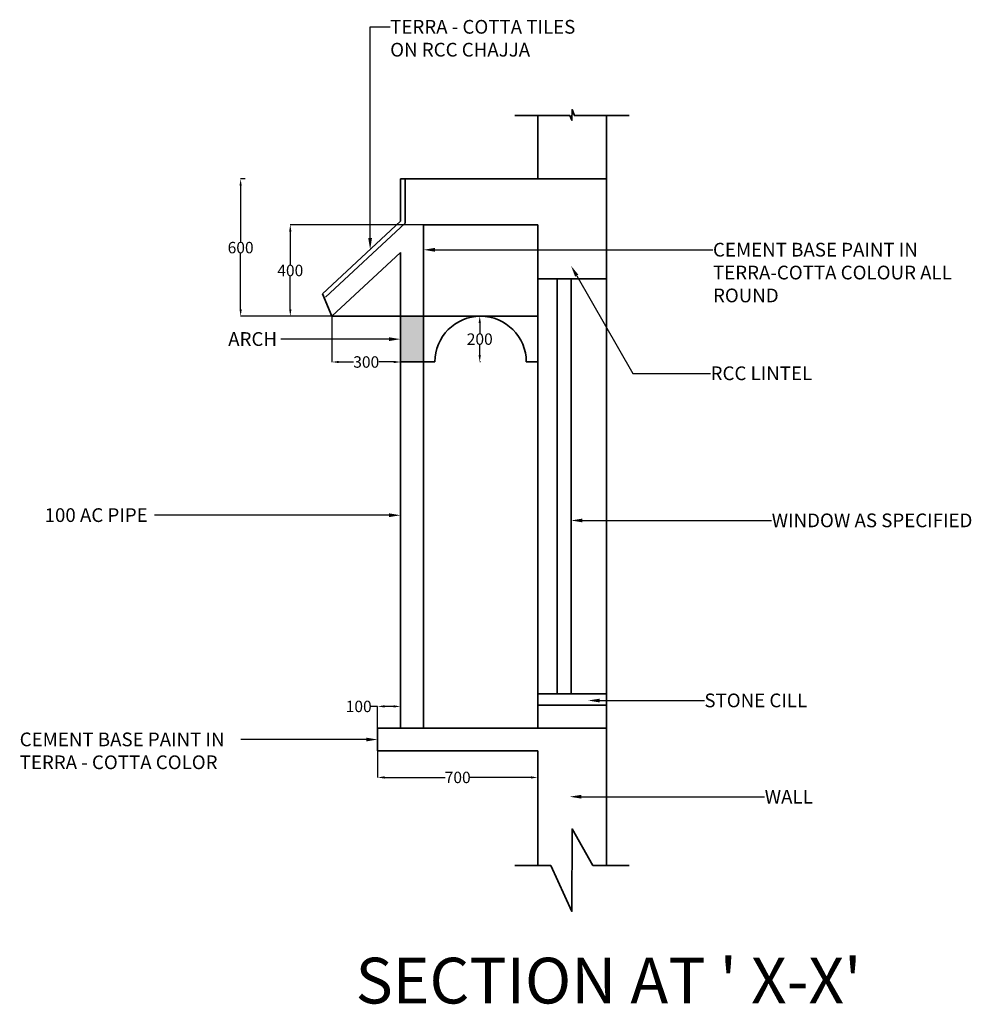
# Model space of a CAD drawing. Units: millimetres. Extents: x 12559 to 31551, y 33148 to 41181.
# Tile 2 of 3: x 19003 to 23164, y 35976 to 40279. Entities that reach past the tile are written whole.
import ezdxf
from ezdxf import colors
from ezdxf.entities.mleader import LeaderData, LeaderLine
from ezdxf.math import Vec2, Vec3

# ---------------------------------------------------------------- set-up
doc = ezdxf.new("R2010")
doc.units = ezdxf.units.MM
doc.header["$MEASUREMENT"] = 0
for name, color, linetype, lineweight in [('A-ANNO-DIMS', 2, 'Continuous', 18), ('A-ANNO-TEXT', 3, 'Continuous', 25), ('A-DETL-PATT', 8, 'Continuous', 13), ('A-SECT', 7, 'Continuous', 35)]:
    doc.layers.add(name, color=color, linetype=linetype, lineweight=lineweight)
doc.styles.get("Standard").update_dxf_attribs({"font": 'arial.ttf'})
doc.dimstyles.get("Standard").update_dxf_attribs({"dimtxt": 100, "dimasz": 0.18, "dimexe": 0.18, "dimexo": 0.0625, "dimgap": 0.09, "dimtad": 0, "dimtih": 1, "dimtoh": 1, "dimdec": 0, "dimzin": 0, "dimdsep": 46, "dimtxsty": 'Standard', "dimcen": 0.09, "dimadec": 0, "dimazin": 0, "dimtfac": 1, "dimtdec": 0, "dimtofl": 0, "dimtmove": 0, "dimatfit": 3, "dimfxl": 1, "dimtolj": 1, "dimtzin": 0, "dimarcsym": 0})

# ---------------------------------------------------------------- blocks, each defined once
blk = doc.blocks.new('*D24')
at = {"layer": 'A-ANNO-DIMS', "color": 0, "lineweight": -2, "transparency": 16777216}
for p, q in [((21018, 38983.1), (21014.3, 38983.1)), ((21014.5, 38953.1), (21014.5, 38908.7)), ((21014.5, 38813.1), (21014.5, 38857.4)), ((21018, 38783.1), (21014.3, 38783.1))]:
    blk.add_line(p, q, dxfattribs=at)
at = {"layer": 'A-ANNO-DIMS', "color": 0, "transparency": 16777216}
for points in [[(21009.5, 38953.1), (21019.5, 38953.1), (21014.5, 38983.1)], [(21009.5, 38813.1), (21019.5, 38813.1), (21014.5, 38783.1)]]:
    blk.add_solid(points, dxfattribs=at)
at = {"layer": 'DEFPOINTS', "color": 0, "transparency": 16777216}
for p in [(21018.1, 38983.1), (21014.5, 38783.1), (21018.1, 38783.1)]:
    blk.add_point(p, dxfattribs=at)
at = {"layer": 'A-ANNO-DIMS', "color": 0, "transparency": 16777216, "insert": (21014.5, 38883.1), "char_height": 50, "attachment_point": 5}
blk.add_mtext('\\A1;200', dxfattribs=at)
blk = doc.blocks.new('*D25')
at = {"layer": 'A-ANNO-DIMS', "color": 0, "lineweight": -2, "transparency": 16777216}
for p, q in [((20368.1, 38983), (20368.1, 38782.9)), ((20668.1, 38983), (20668.1, 38782.9)), ((20398.1, 38783.1), (20462.8, 38783.1)), ((20638.1, 38783.1), (20573.3, 38783.1))]:
    blk.add_line(p, q, dxfattribs=at)
at = {"layer": 'A-ANNO-DIMS', "color": 0, "transparency": 16777216}
for points in [[(20398.1, 38788.1), (20398.1, 38778.1), (20368.1, 38783.1)], [(20638.1, 38788.1), (20638.1, 38778.1), (20668.1, 38783.1)]]:
    blk.add_solid(points, dxfattribs=at)
at = {"layer": 'DEFPOINTS', "color": 0, "transparency": 16777216}
for p in [(20368.1, 38983.1), (20668.1, 38983.1), (20668.1, 38783.1)]:
    blk.add_point(p, dxfattribs=at)
at = {"layer": 'A-ANNO-DIMS', "color": 0, "transparency": 16777216, "insert": (20518.1, 38783.1), "char_height": 50, "attachment_point": 5}
blk.add_mtext('\\A1;300', dxfattribs=at)
blk = doc.blocks.new('*D26')
at = {"layer": 'A-ANNO-DIMS', "color": 0, "lineweight": -2, "transparency": 16777216}
for p, q in [((20768, 39383.1), (20185.8, 39383.1)), ((20186, 39353.1), (20186, 39208.7)), ((20186, 39013.1), (20186, 39157.4)), ((20768, 38983.1), (20185.8, 38983.1))]:
    blk.add_line(p, q, dxfattribs=at)
at = {"layer": 'A-ANNO-DIMS', "color": 0, "transparency": 16777216}
for points in [[(20181, 39353.1), (20191, 39353.1), (20186, 39383.1)], [(20181, 39013.1), (20191, 39013.1), (20186, 38983.1)]]:
    blk.add_solid(points, dxfattribs=at)
at = {"layer": 'DEFPOINTS', "color": 0, "transparency": 16777216}
for p in [(20186, 39383.1), (20768.1, 39383.1), (20768.1, 38983.1)]:
    blk.add_point(p, dxfattribs=at)
at = {"layer": 'A-ANNO-DIMS', "color": 0, "transparency": 16777216, "insert": (20186, 39183.1), "char_height": 50, "attachment_point": 5}
blk.add_mtext('\\A1;400', dxfattribs=at)
blk = doc.blocks.new('*D27')
at = {"layer": 'A-ANNO-DIMS', "color": 0, "lineweight": -2, "transparency": 16777216}
for p, q in [((19988.8, 39583.1), (19968.6, 39583.1)), ((19968.8, 39553.1), (19968.8, 39308.7)), ((19968.8, 39013.1), (19968.8, 39257.4)), ((20185.7, 38983.1), (19968.6, 38983.1))]:
    blk.add_line(p, q, dxfattribs=at)
at = {"layer": 'A-ANNO-DIMS', "color": 0, "transparency": 16777216}
for points in [[(19963.8, 39553.1), (19973.8, 39553.1), (19968.8, 39583.1)], [(19963.8, 39013.1), (19973.8, 39013.1), (19968.8, 38983.1)]]:
    blk.add_solid(points, dxfattribs=at)
at = {"layer": 'DEFPOINTS', "color": 0, "transparency": 16777216}
for p in [(19988.8, 39583.1), (19968.8, 38983.1), (20185.8, 38983.1)]:
    blk.add_point(p, dxfattribs=at)
at = {"layer": 'A-ANNO-DIMS', "color": 0, "transparency": 16777216, "insert": (19968.8, 39283.1), "char_height": 50, "attachment_point": 5}
blk.add_mtext('\\A1;600', dxfattribs=at)
blk = doc.blocks.new('*D28')
at = {"layer": 'A-ANNO-DIMS', "color": 0, "lineweight": -2, "transparency": 16777216}
for p, q in [((20568.1, 37083), (20568.1, 36967.2)), ((21268.1, 37083), (21268.1, 36967.2)), ((20598.1, 36967.4), (20863, 36967.4)), ((21238.1, 36967.4), (20973.1, 36967.4))]:
    blk.add_line(p, q, dxfattribs=at)
at = {"layer": 'A-ANNO-DIMS', "color": 0, "transparency": 16777216}
for points in [[(20598.1, 36972.4), (20598.1, 36962.4), (20568.1, 36967.4)], [(21238.1, 36972.4), (21238.1, 36962.4), (21268.1, 36967.4)]]:
    blk.add_solid(points, dxfattribs=at)
at = {"layer": 'DEFPOINTS', "color": 0, "transparency": 16777216}
for p in [(20568.1, 37083.1), (21268.1, 37083.1), (21268.1, 36967.4)]:
    blk.add_point(p, dxfattribs=at)
at = {"layer": 'A-ANNO-DIMS', "color": 0, "transparency": 16777216, "insert": (20918.1, 36967.4), "char_height": 50, "attachment_point": 5}
blk.add_mtext('\\A1;700', dxfattribs=at)
blk = doc.blocks.new('*D29')
at = {"layer": 'A-ANNO-DIMS', "color": 0, "lineweight": -2, "transparency": 16777216}
for p, q in [((20568.1, 37277.8), (20538.1, 37277.8)), ((20568.1, 37183.1), (20568.1, 37278)), ((20638.1, 37277.8), (20598.1, 37277.8)), ((20668.1, 37183.1), (20668.1, 37278))]:
    blk.add_line(p, q, dxfattribs=at)
at = {"layer": 'A-ANNO-DIMS', "color": 0, "transparency": 16777216}
for points in [[(20598.1, 37282.8), (20598.1, 37272.8), (20568.1, 37277.8)], [(20638.1, 37282.8), (20638.1, 37272.8), (20668.1, 37277.8)]]:
    blk.add_solid(points, dxfattribs=at)
at = {"layer": 'DEFPOINTS', "color": 0, "transparency": 16777216}
for p in [(20568.1, 37277.8), (20568.1, 37183.1), (20668.1, 37183.1)]:
    blk.add_point(p, dxfattribs=at)
at = {"layer": 'A-ANNO-DIMS', "color": 0, "transparency": 16777216, "insert": (20485.2, 37277.8), "char_height": 50, "attachment_point": 5}
blk.add_mtext('\\A1;100', dxfattribs=at)

msp = doc.modelspace()

# ---------------------------------------------------------------- hatches: boundary and pattern name
at = {"layer": 'A-DETL-PATT'}
h = msp.add_hatch(color=256, dxfattribs=at)
h.dxf.hatch_style = 1
h.paths.add_polyline_path([(20668.1, 38783.1), (20768.1, 38783.1), (20768.1, 38983.1), (20668.1, 38983.1)])

# ---------------------------------------------------------------- linework, layer by layer
at = {"layer": 'A-SECT'}
for p, q in [((21267.9, 39860.4), (21167.9, 39860.4)), ((21268.1, 39860.4), (21268.1, 39583.1)), ((21268.1, 39860.4), (21408.3, 39860.4)), ((21428.5, 39860.4), (21568.1, 39860.4)), ((21568.1, 39860.4), (21568.1, 36583.1)), ((21568.1, 39860.4), (21668.1, 39860.4)), ((21568.1, 39583.1), (20668.1, 39583.1)), ((20668.1, 39398), (20668.1, 39583.1)), ((20688.1, 39389.3), (20688.1, 39583.1)), ((20326.8, 39081.2), (20668.1, 39398)), ((20340.4, 39066.6), (20688.1, 39389.3)), ((20768.1, 37183.1), (20768.1, 39383.1)), ((21268.1, 39383.1), (20768.1, 39383.1)), ((21268.1, 39383.1), (21268.1, 37183.1)), ((20368.1, 38983.1), (20668.1, 39261.6)), ((20668.1, 37183.1), (20668.1, 39261.6)), ((21268.1, 39146.1), (21568.1, 39146.1)), ((21353.8, 39146.1), (21353.8, 37333.1)), ((21413.8, 39146.1), (21413.8, 37333.1)), ((20368.1, 38983.1), (20326.8, 39081.2)), ((20668.1, 38983.1), (20368.1, 38983.1)), ((21268.1, 38983.1), (20668.1, 38983.1)), ((20818.1, 38783.1), (20668.1, 38783.1)), ((20768.1, 38783.1), (20818.1, 38783.1)), ((21268.1, 38783.1), (21218.1, 38783.1)), ((21218.1, 38783.1), (21268.1, 38783.1)), ((21568.1, 37333.1), (21268.1, 37333.1)), ((21568.1, 37283.1), (21268.1, 37283.1)), ((21568.1, 37183.1), (20568.1, 37183.1)), ((20568.1, 37183.1), (20568.1, 37083.1)), ((21268.1, 37083.1), (20568.1, 37083.1)), ((21268.1, 37083.1), (21268.1, 36583.1)), ((21268.1, 36583.1), (21168.1, 36583.1)), ((21268.1, 36583.1), (21324.9, 36583.1)), ((21509.5, 36583.1), (21568.1, 36583.1)), ((21568.1, 36583.1), (21668.1, 36583.1))]:
    msp.add_line(p, q, dxfattribs=at)
for points in [[(21267.9, 39860.4), (21408.3, 39860.4), (21417.9, 39839.6), (21418.2, 39886.3), (21428.5, 39860.4), (21568.2, 39860.4)], [(20668.1, 38687.7), (20668.1, 38983.1), (20768.1, 38983.1), (20768.1, 38687.7)], [(21267.9, 36583.1), (21324.9, 36583.1), (21417.9, 36381.6), (21418.2, 36742.3), (21509.5, 36583.1), (21568.2, 36583.1)]]:
    msp.add_lwpolyline(points, dxfattribs=at)
msp.add_arc((21018.1, 38783.1), 200, 0, 180, dxfattribs=at)

# ---------------------------------------------------------------- texts
at = {"layer": 'A-ANNO-TEXT', "insert": (20471.5, 36179.4), "char_height": 200, "attachment_point": 1}
msp.add_mtext_dynamic_manual_height_columns("SECTION AT ' X-X'", width=3493.58, gutter_width=1, heights=[0], dxfattribs=at)

# ---------------------------------------------------------------- dimensions: what is measured, and where the dimension line sits
at = {"layer": 'A-ANNO-DIMS'}
for base, p1, p2, picture, middle in [((19968.8, 38983.1), (19988.8, 39583.1), (20185.8, 38983.1), '*D27', (19968.8, 39283.1)), ((20186, 39383.1), (20768.1, 38983.1), (20768.1, 39383.1), '*D26', (20186, 39183.1)), ((21014.5, 38783.1), (21018.1, 38983.1), (21018.1, 38783.1), '*D24', (21014.5, 38883.1))]:
    dim = msp.add_linear_dim(base=base, p1=p1, p2=p2, angle=90, dimstyle='Standard', override={"dimtxt": 50, "dimasz": 30, "dimclrd": 0, "dimclre": 0, "dimclrt": 0}, dxfattribs=at)
    dim.commit()
    dim.dimension.update_dxf_attribs({"geometry": picture, "text_midpoint": middle})
for base, p1, p2, picture, middle in [((20668.1, 38783.1), (20368.1, 38983.1), (20668.1, 38983.1), '*D25', (20518.1, 38783.1)), ((20568.1, 37277.8), (20668.1, 37183.1), (20568.1, 37183.1), '*D29', (20485.2, 37277.8)), ((21268.1, 36967.4), (20568.1, 37083.1), (21268.1, 37083.1), '*D28', (20918.1, 36967.4))]:
    dim = msp.add_linear_dim(base=base, p1=p1, p2=p2, dimstyle='Standard', override={"dimtxt": 50, "dimasz": 30, "dimclrd": 0, "dimclre": 0, "dimclrt": 0}, dxfattribs=at)
    dim.commit()
    dim.dimension.update_dxf_attribs({"geometry": picture, "text_midpoint": middle})

# ---------------------------------------------------------------- leaders
at = {"layer": 'A-ANNO-TEXT'}
ml = msp.add_multileader_mtext('Standard', dxfattribs=at)
ml.set_content('TERRA - COTTA TILES \\PON RCC CHAJJA', color=256)
ml.set_leader_properties()
ml.build(insert=Vec2(0, 0))
ml.multileader.update_dxf_attribs({"dogleg_length": 0.36, "arrow_head_size": 50})
ctx = ml.context
ctx.base_point, ctx.char_height, ctx.arrow_head_size, ctx.landing_gap_size, ctx.plane_origin = Vec3(20622.7, 40247.6), 60, 50, 0.09, Vec3(20535.1, 39274.6)
notes = []
notes.append((ctx, [(0, (1, 1, 0), (20535.1, 40247.6), (1, 0), 87.6, [(0, [(20535.1, 39274.6)], 0, [])])]))
ctx.mtext.insert, ctx.mtext.flow_direction = Vec3(20622.8, 40278.1), 5
ml = msp.add_multileader_mtext('Standard', dxfattribs=at)
ml.set_content('CEMENT BASE PAINT IN\\PTERRA-COTTA COLOUR ALL\\PROUND', color=256)
ml.set_leader_properties()
ml.build(insert=Vec2(0, 0))
ml.multileader.update_dxf_attribs({"dogleg_length": 87.6, "arrow_head_size": 50})
ctx = ml.context
ctx.base_point, ctx.char_height, ctx.arrow_head_size, ctx.landing_gap_size, ctx.plane_origin = Vec3(22034.5, 39273.5), 60, 50, 0.09, Vec3(20768.1, 39273.5)
notes.append((ctx, [(0, (1, 1, 0), (21946.8, 39273.5), (1, 0), 87.6, [(0, [(20768.1, 39273.5)], 0, [])])]))
ctx.mtext.insert, ctx.mtext.flow_direction = Vec3(22034.5, 39304), 5
ml = msp.add_multileader_mtext('Standard', dxfattribs=at)
ml.set_content('RCC LINTEL', color=256)
ml.set_leader_properties()
ml.build(insert=Vec2(0, 0))
ml.multileader.update_dxf_attribs({"dogleg_length": 87.6, "arrow_head_size": 50})
ctx = ml.context
ctx.base_point, ctx.char_height, ctx.arrow_head_size, ctx.landing_gap_size, ctx.plane_origin = Vec3(22024, 38733.3), 60, 50, 0.09, Vec3(21413.8, 39203.5)
notes.append((ctx, [(0, (1, 1, 0), (21684.1, 38733.3), (1, 0), 339.9, [(0, [(21413.8, 39203.5)], 0, [])])]))
ctx.mtext.insert, ctx.mtext.flow_direction = Vec3(22024.1, 38763.8), 5
ml = msp.add_multileader_mtext('Standard', dxfattribs=at)
ml.set_content('ARCH', color=256)
ml.set_leader_properties()
ml.build(insert=Vec2(0, 0))
ml.multileader.update_dxf_attribs({"dogleg_length": 87.6, "arrow_head_size": 50})
ctx = ml.context
ctx.base_point, ctx.char_height, ctx.arrow_head_size, ctx.landing_gap_size, ctx.plane_origin = Vec3(19914.4, 38882.9), 60, 50, 0.09, Vec3(20668.1, 38882.9)
notes.append((ctx, [(0, (1, 1, 0), (20232.9, 38882.9), (-1, 0), 87.6, [(0, [(20668.1, 38882.9)], 0, [])])]))
ctx.mtext.insert, ctx.mtext.flow_direction = Vec3(19914.5, 38913.5), 5
ml = msp.add_multileader_mtext('Standard', dxfattribs=at)
ml.set_content('100 AC PIPE', color=256)
ml.set_leader_properties()
ml.build(insert=Vec2(0, 0))
ml.multileader.update_dxf_attribs({"dogleg_length": 339.9, "arrow_head_size": 50})
ctx = ml.context
ctx.base_point, ctx.char_height, ctx.arrow_head_size, ctx.landing_gap_size, ctx.plane_origin = Vec3(19111.4, 38113.4), 60, 50, 0.09, Vec3(20668.1, 38113.4)
notes.append((ctx, [(0, (1, 1, 0), (19931.8, 38113.4), (-1, 0), 339.9, [(0, [(20668.1, 38113.4)], 0, [])])]))
ctx.mtext.insert, ctx.mtext.flow_direction = Vec3(19111.5, 38143.9), 5
ml = msp.add_multileader_mtext('Standard', dxfattribs=at)
ml.set_content('WINDOW AS SPECIFIED', color=256)
ml.set_leader_properties()
ml.build(insert=Vec2(0, 0))
ml.multileader.update_dxf_attribs({"dogleg_length": 339.9, "arrow_head_size": 50})
ctx = ml.context
ctx.base_point, ctx.char_height, ctx.arrow_head_size, ctx.landing_gap_size, ctx.plane_origin = Vec3(22291, 38090.4), 60, 50, 0.09, Vec3(21413.8, 38090.4)
notes.append((ctx, [(0, (1, 1, 0), (21951.1, 38090.4), (1, 0), 339.9, [(0, [(21413.8, 38090.4)], 0, [])])]))
ctx.mtext.insert, ctx.mtext.flow_direction = Vec3(22291.1, 38120.9), 5
ml = msp.add_multileader_mtext('Standard', dxfattribs=at)
ml.set_content('STONE CILL', color=256)
ml.set_leader_properties()
ml.build(insert=Vec2(0, 0))
ml.multileader.update_dxf_attribs({"dogleg_length": 339.9, "arrow_head_size": 50})
ctx = ml.context
ctx.base_point, ctx.char_height, ctx.arrow_head_size, ctx.landing_gap_size, ctx.plane_origin = Vec3(21996.8, 37303.5), 60, 50, 0.09, Vec3(21488.8, 37303.5)
notes.append((ctx, [(0, (1, 1, 0), (21656.8, 37303.5), (1, 0), 339.9, [(0, [(21488.8, 37303.5)], 0, [])])]))
ctx.mtext.insert, ctx.mtext.flow_direction = Vec3(21996.9, 37334), 5
ml = msp.add_multileader_mtext('Standard', dxfattribs=at)
ml.set_content('CEMENT BASE PAINT IN\\PTERRA - COTTA COLOR', color=256)
ml.set_leader_properties()
ml.build(insert=Vec2(0, 0))
ml.multileader.update_dxf_attribs({"dogleg_length": 339.9, "arrow_head_size": 50})
ctx = ml.context
ctx.base_point, ctx.char_height, ctx.arrow_head_size, ctx.landing_gap_size, ctx.plane_origin = Vec3(19002.5, 37133.1), 60, 50, 0.09, Vec3(20568.1, 37133.1)
notes.append((ctx, [(0, (1, 1, 0), (20309.6, 37133.1), (-1, 0), 339.9, [(0, [(20568.1, 37133.1)], 0, [])])]))
ctx.mtext.insert, ctx.mtext.flow_direction = Vec3(19002.6, 37163.6), 5
ml = msp.add_multileader_mtext('Standard', dxfattribs=at)
ml.set_content('WALL', color=256)
ml.set_leader_properties()
ml.build(insert=Vec2(0, 0))
ml.multileader.update_dxf_attribs({"dogleg_length": 339.9, "arrow_head_size": 50})
ctx = ml.context
ctx.base_point, ctx.char_height, ctx.arrow_head_size, ctx.landing_gap_size, ctx.plane_origin = Vec3(22260.4, 36883.1), 60, 50, 0.09, Vec3(21408.1, 36883.1)
notes.append((ctx, [(0, (1, 1, 0), (21920.5, 36883.1), (1, 0), 339.9, [(0, [(21408.1, 36883.1)], 0, [])])]))
ctx.mtext.insert, ctx.mtext.flow_direction = Vec3(22260.5, 36913.1), 5
for ctx, leaders in notes:
    for number, flags, end, landing, length, lines in leaders:
        leader = LeaderData()
        leader.index, (leader.has_last_leader_line, leader.has_dogleg_vector, leader.attachment_direction) = number, flags
        leader.last_leader_point, leader.dogleg_vector, leader.dogleg_length = Vec3(end), Vec3(landing), length
        for number, points, colour, breaks in lines:
            line = LeaderLine()
            line.index, line.vertices, line.color, line.breaks = number, Vec3.list(points), colors.encode_raw_color(colour), breaks
            leader.lines.append(line)
        ctx.leaders.append(leader)

doc.saveas('drawing.dxf')
